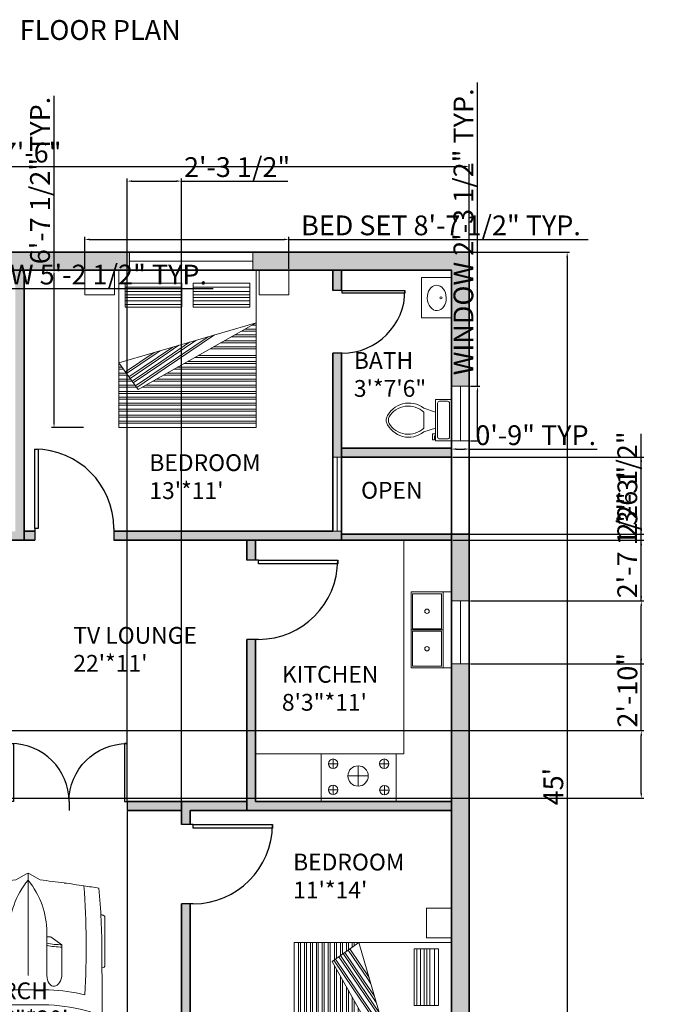
# Model space of a CAD drawing. Units: inches. Extents: x 1698 to 2352, y 1975 to 2732.
# Tile 4 of 4: x 2029 to 2352, y 2234 to 2732. Entities that reach past the tile are written whole.
import ezdxf

# ---------------------------------------------------------------- set-up
doc = ezdxf.new("R2010")
doc.units = ezdxf.units.IN
for name, color, linetype, lineweight in [('A-ANNO-DIMS', 2, 'Continuous', 18), ('A-ANNO-TEXT', 7, 'Continuous', 25), ('A-AREA-IDEN', 7, 'Continuous', 18), ('A-EQPM', 10, 'Continuous', 18), ('A-FLOR-CASE', 9, 'Continuous', 18), ('A-FLOR-FIXT', 231, 'Continuous', 18), ('A-WALL-PATT', 52, 'Continuous', 13), ('car', 171, 'Continuous', 13), ('door', 80, 'Continuous', 25), ('fur', 10, 'Continuous', 18), ('wall', 7, 'Continuous', 35), ('window', 130, 'Continuous', 18)]:
    doc.layers.add(name, color=color, linetype=linetype, lineweight=lineweight)
doc.styles.get("Standard").update_dxf_attribs({"font": 'arial.ttf'})
doc.dimstyles.new('ISO-25', dxfattribs={"dimtxt": 10, "dimasz": 2.5, "dimexe": 1.25, "dimexo": 0.625, "dimtad": 1, "dimdec": 0, "dimlunit": 4, "dimtxsty": 'Standard', "dimcen": 2.5, "dimadec": 0, "dimazin": 0, "dimtfac": 1, "dimtdec": 0, "dimtmove": 0, "dimatfit": 3, "dimfxl": 1, "dimarcsym": 0})

# ---------------------------------------------------------------- blocks, each defined once
blk = doc.blocks.new('*U2')
for p, q in [((0, 0), (0, -6)), ((40, 0), (40, -6))]:
    blk.add_line(p, q)
blk.add_lwpolyline([(0, 0), (0, 40), (1.75, 40), (1.75, 0)], close=True)
blk.add_arc((0, 0), 40, 0, 90)
blk = doc.blocks.new('*U6')
for p, q in [((21.1, 37.41), (21.1, 36.83)), ((46.55, 38.89), (22.35, 38.89)), ((47.8, 37.39), (47.8, 37.41)), ((87.99, 31.87), (74.76, 35.92)), ((134.31, 35.6), (119.29, 31.78)), ((135.45, 37.07), (135.45, 37.41)), ((136.7, 38.89), (160.9, 38.89)), ((162.15, 37.41), (162.15, 36.77)), ((70.03, 31.54), (86.41, 29.35)), ((186.47, -33.5), (186.47, 33.5)), ((188.4, -32.76), (188.4, 32.76)), ((138.42, 29.35), (157.25, 29.35)), ((164.52, 26.39), (164.52, -26.39)), ((186.47, 29.35), (167.01, 29.35)), ((32.27, 11.63), (36.13, 17.17)), ((36.13, 17.17), (50.94, 17.17)), ((32.12, 9.51), (32.12, 11.15)), ((58.92, -10.77), (58.92, 10.77)), ((66.55, -10.53), (66.55, 10.53)), ((186.47, -10.53), (186.47, 10.53)), ((3.27, 6.13), (0.1, 0.41)), ((29.77, 9.51), (51.68, 9.51)), ((82.74, 8.5), (82.74, -8.5)), ((0, 0), (51.68, 0)), ((0.1, -0.41), (3.27, -6.13)), ((29.77, -9.51), (51.68, -9.51)), ((32.12, -9.51), (32.12, -11.15)), ((32.27, -11.63), (36.13, -17.17)), ((36.13, -17.17), (50.94, -17.17)), ((86.41, -29.35), (70.03, -31.54)), ((157.25, -29.35), (138.42, -29.35)), ((167.01, -29.35), (186.47, -29.35)), ((87.99, -31.87), (74.76, -35.92)), ((134.31, -35.6), (119.29, -31.78)), ((21.1, -37.41), (21.1, -36.83)), ((46.55, -38.89), (22.35, -38.89)), ((47.8, -37.39), (47.8, -37.41)), ((135.45, -37.07), (135.45, -37.41)), ((136.7, -38.89), (160.9, -38.89)), ((162.15, -37.41), (162.15, -36.77))]:
    blk.add_line(p, q)
for centre, major_axis, ratio, start_param, end_param in [((266.03, -27.52), (0, 313.31), 0.842304, 1.367076, 1.39176), ((41.19, -490.86), (0, 528.23), 0.842304, 0.00281, 0.075598), ((22.35, 37.41), (0, -1.48), 0.842304, 3.141593, 4.712389), ((64.48, -10555.62), (0, 10593.03), 0.842304, -0.013397, 0.002797), ((46.55, 37.41), (0, 1.48), 0.842304, -1.570796, 0), ((64.48, -10555.62), (0, -10591.55), 0.842304, 3.133765, 3.140441), ((136.7, 37.41), (0, -1.48), 0.842304, 3.141593, 4.712389), ((160.9, 37.41), (0, 1.48), 0.842304, -1.570796, 0), ((180.63, 35.84), (0, 2.22), 0.842304, -0.013017, 1.249894), ((64.48, -10556.36), (0, 10595.31), 0.842304, -0.013397, -0.013017), ((183.98, 33.5), (0, -2.96), 0.842304, 1.570796, 3.128196), ((183.98, 32.76), (0, -5.25), 0.842304, 1.570796, 3.128196), ((135.29, 5.39), (0, 81.77), 0.842304, 1.245306, 1.50788), ((95.79, -3666.35), (0, -3698.24), 0.842304, 3.134049, 3.144098), ((259.18, -27.52), (0, -305.3), 0.842304, 4.528606, 4.561838), ((37.47, -593.96), (0, -623.33), 0.842304, 3.096046, 3.200911), ((134.4, 5.39), (0, -89.78), 0.842304, 4.449482, 4.652344), ((149.6, 2.8), (0, -79.58), 0.842304, 4.372215, 4.640744), ((17.08, 0), (0, 147.02), 0.842304, 4.511394, 4.913384), ((35.91, 0), (0, 147.02), 0.842304, 4.511394, 4.913384), ((167.01, 26.39), (0, 2.96), 0.842304, 0, 1.570796), ((-204.49, 52.4), (0, -250.96), 0.842304, 1.385369, 1.434372), ((13.04, 17.01), (0, 27.42), 0.842304, 4.435146, 4.718221), ((14.2, 17.01), (0, 27.42), 0.842304, 4.435146, 4.718221), ((50.79, 13.34), (6.34, -0.36), 0.603834, -1.395552, 1.581315), ((32.75, 11.15), (0, 0.74), 0.842304, 0.879714, 1.570796), ((29.77, -46.66), (0, 56.17), 0.842304, 0, 0.590319), ((0.62, 0), (0, -0.74), 0.842304, 4.131459, 5.293319), ((29.77, 46.66), (0, 56.17), 0.842304, 2.551274, 3.141593), ((-204.49, -52.4), (0, 250.96), 0.842304, -1.434372, -1.385369), ((13.04, -17.01), (0, -27.42), 0.842304, 1.564964, 1.848039), ((14.2, -17.01), (0, -27.42), 0.842304, 1.564964, 1.848039), ((149.6, -2.8), (0, -79.58), 0.842304, -1.499151, -1.230623), ((32.75, -11.15), (0, -0.74), 0.842304, 4.712389, 5.403472), ((134.4, -5.39), (0, -89.78), 0.842304, -1.510751, -1.307889), ((135.29, -5.39), (0, -81.77), 0.842304, -1.50788, -1.245306), ((259.18, 27.52), (0, 305.3), 0.842304, 1.721348, 1.754579), ((266.03, 27.52), (0, 313.31), 0.842304, 1.749832, 1.774517), ((37.47, 593.96), (0, -623.33), 0.842304, -0.059319, 0.045547), ((167.01, -26.39), (0, -2.96), 0.842304, 4.712389, 6.283185), ((95.79, 3666.35), (0, -3698.24), 0.842304, -0.002505, 0.007544), ((183.98, -33.5), (0, 2.96), 0.842304, 3.15499, 4.712389), ((183.98, -32.76), (0, -5.25), 0.842304, 0.013397, 1.570796), ((41.19, 490.86), (0, -528.23), 0.842304, -0.075598, -0.00281), ((22.35, -37.41), (0, 1.48), 0.842304, 1.570796, 3.141593), ((64.48, 10555.62), (0, 10593.03), 0.842304, 3.138796, 3.15499), ((46.55, -37.41), (0, -1.48), 0.842304, 0, 1.570796), ((64.48, 10555.62), (0, -10591.55), 0.842304, 0.001152, 0.007828), ((136.7, -37.41), (0, -1.48), 0.842304, -1.570796, 0), ((160.9, -37.41), (0, 1.48), 0.842304, 3.141593, 4.712389), ((180.63, -35.84), (0, -2.22), 0.842304, -1.249894, 0.013017), ((64.48, 10556.36), (0, 10595.31), 0.842304, 3.15461, 3.15499)]:
    blk.add_ellipse(centre, major_axis=major_axis, ratio=ratio, start_param=start_param, end_param=end_param)
at = {"extrusion": (0, 0, -1)}
blk.add_ellipse((50.79, -13.34), major_axis=(6.34, 0.36), ratio=0.603834, start_param=-1.395552, end_param=1.581315, dxfattribs=at)
blk = doc.blocks.new('*U4')
for p, q in [((9.5, -6), (9.5, -2)), ((-10, -8.5), (-8, -8.5)), ((-10, -9.5), (-10, -8.5)), ((-7, -9.5), (-10, -9.5)), ((-8, -8.5), (-8, -8)), ((-7, -8), (-7, -9.5)), ((-4, -8), (-6, -14)), ((4, -8), (6, -14)), ((4, -14), (-4, -14))]:
    blk.add_line(p, q)
blk.add_lwpolyline([(10.5, -8), (10.5, 0), (-10.5, 0), (-10.5, -8)], close=True)
for points in [[(-9.5, -2), (-9.5, -6)], [(8.5, -1), (-8.5, -1)], [(-8.5, -7), (8.5, -7)]]:
    blk.add_lwpolyline(points)
for centre, radius, start, end in [((-8.62, -1.88), 0.884, 81.8699, 188.1301), ((8.62, -1.88), 0.884, 351.8699, 98.1301), ((-8.62, -6.12), 0.884, 171.8699, 278.1301), ((8.62, -6.12), 0.884, 261.8699, 8.1301), ((3.52, -21.58), 12.17, 141.4691, 247.9714), ((4.2, -21.82), 11.33, 136.3677, 238.9468), ((-3.52, -21.58), 12.17, 292.0284, 38.5307), ((-4.2, -21.82), 11.33, 301.053, 43.6321), ((0, -27.88), 4, 245.7318, 294.2682), ((0, -29), 4, 254.8605, 285.1395)]:
    blk.add_arc(centre, radius, start, end)
blk = doc.blocks.new('*D7')
at = {"layer": 'A-ANNO-DIMS', "color": 0, "lineweight": -2, "transparency": 16777216}
for p, q in [((1805.99, 2614.89), (1805.99, 2658.85)), ((1808.49, 2657.6), (2253.49, 2657.6)), ((2255.99, 2614.89), (2255.99, 2658.85))]:
    blk.add_line(p, q, dxfattribs=at)
at = {"layer": 'A-ANNO-DIMS', "color": 0, "lineweight": 100, "transparency": 16777216}
for points in [[(1808.49, 2658.02), (1808.49, 2657.18), (1805.99, 2657.6)], [(2253.49, 2658.02), (2253.49, 2657.18), (2255.99, 2657.6)]]:
    blk.add_solid(points, dxfattribs=at)
at = {"layer": 'Defpoints', "color": 0, "lineweight": 100, "transparency": 16777216}
for p in [(2255.99, 2657.6), (1805.99, 2614.26), (2255.99, 2614.26)]:
    blk.add_point(p, dxfattribs=at)
at = {"layer": 'A-ANNO-DIMS', "color": 0, "transparency": 16777216, "insert": (2030.99, 2663.33), "char_height": 10, "attachment_point": 5}
blk.add_mtext('37\'-6"', dxfattribs=at)
blk = doc.blocks.new('*D8')
at = {"layer": 'A-ANNO-DIMS', "color": 0, "lineweight": -2, "transparency": 16777216}
for p, q in [((2256.62, 2614.26), (2306.74, 2614.26)), ((2305.49, 2611.76), (2305.49, 2076.76)), ((2256.62, 2074.26), (2306.74, 2074.26))]:
    blk.add_line(p, q, dxfattribs=at)
at = {"layer": 'A-ANNO-DIMS', "color": 0, "lineweight": 100, "transparency": 16777216}
for points in [[(2305.07, 2611.76), (2305.9, 2611.76), (2305.49, 2614.26)], [(2305.07, 2076.76), (2305.9, 2076.76), (2305.49, 2074.26)]]:
    blk.add_solid(points, dxfattribs=at)
at = {"layer": 'Defpoints', "color": 0, "lineweight": 100, "transparency": 16777216}
for p in [(2255.99, 2614.26), (2255.99, 2074.26), (2305.49, 2074.26)]:
    blk.add_point(p, dxfattribs=at)
at = {"layer": 'A-ANNO-DIMS', "color": 0, "transparency": 16777216, "insert": (2299.78, 2344.26), "char_height": 10, "attachment_point": 5, "rotation": 90}
blk.add_mtext("45'", dxfattribs=at)
blk = doc.blocks.new('BED-DOUBLE-WITH-NIGHTSTANDS')
for p, q in [((20.55, 70.98), (49.18, 70.98)), ((54.81, 70.98), (83.45, 70.98)), ((20.55, 67.05), (49.18, 67.05)), ((20.55, 65.74), (49.18, 65.74)), ((20.61, 68.69), (49.25, 68.69)), ((54.81, 67.05), (83.45, 67.05)), ((54.81, 65.74), (83.45, 65.74)), ((54.87, 68.69), (83.51, 68.69)), ((20.55, 63.98), (49.18, 63.98)), ((20.55, 62.15), (49.18, 62.15)), ((54.81, 63.98), (83.45, 63.98)), ((54.81, 62.15), (83.45, 62.15)), ((17.28, 32.76), (86.63, 52.89)), ((86.63, 52.89), (27, 19.28)), ((81.11, 49.78), (86.63, 49.78)), ((84.66, 51.78), (86.63, 51.78)), ((86.25, 52.78), (86.63, 52.78)), ((40.19, 30.78), (62.43, 45.87)), ((40.75, 29.96), (65.55, 46.77)), ((74.02, 45.78), (86.63, 45.78)), ((75.79, 46.78), (86.63, 46.78)), ((79.34, 48.78), (86.63, 48.78)), ((36.83, 35.44), (44.53, 40.67)), ((37.39, 34.62), (47.65, 41.57)), ((38.42, 33.24), (53.01, 43.13)), ((38.98, 32.41), (56.13, 44.04)), ((65.15, 40.78), (86.63, 40.78)), ((68.7, 42.78), (86.63, 42.78)), ((70.47, 43.78), (86.63, 43.78)), ((20.62, 28.13), (35.05, 37.91)), ((21.18, 27.3), (35.61, 37.09)), ((22.4, 25.66), (36.83, 35.44)), ((35.61, 37.09), (38.16, 38.82)), ((55.69, 35.45), (86.63, 35.45)), ((57.46, 36.45), (86.63, 36.45)), ((63.38, 39.78), (86.63, 39.78)), ((27, 19.28), (17.28, 32.76)), ((17.28, 32.45), (17.5, 32.45)), ((17.28, 30.45), (18.94, 30.45)), ((22.96, 24.83), (37.39, 34.62)), ((23.99, 23.45), (38.42, 33.24)), ((24.55, 22.62), (38.98, 32.41)), ((25.76, 21), (40.19, 30.78)), ((26.32, 20.17), (40.75, 29.96)), ((46.82, 30.45), (86.63, 30.45)), ((50.37, 32.45), (86.63, 32.45)), ((52.14, 33.45), (86.63, 33.45)), ((17.28, 29.45), (19.66, 29.45)), ((17.28, 27.45), (21.11, 27.45)), ((17.28, 26.45), (21.83, 26.45)), ((39.73, 26.45), (86.63, 26.45)), ((41.5, 27.45), (86.63, 27.45)), ((45.05, 29.45), (86.63, 29.45)), ((17.28, 24.45), (23.27, 24.45)), ((17.28, 23.45), (23.99, 23.45)), ((17.28, 21.45), (25.43, 21.45)), ((17.28, 20.45), (26.16, 20.45)), ((29.09, 20.45), (86.63, 20.45)), ((30.86, 21.45), (86.63, 21.45)), ((34.41, 23.45), (86.63, 23.45)), ((36.18, 24.45), (86.63, 24.45)), ((17.28, 18.28), (86.63, 18.28)), ((17.28, 17.28), (86.63, 17.28)), ((17.28, 15.28), (86.63, 15.28)), ((17.28, 14.28), (86.63, 14.28)), ((17.28, 12.28), (86.63, 12.28)), ((17.28, 11.28), (86.63, 11.28)), ((17.28, 9.28), (86.63, 9.28)), ((17.28, 8.28), (86.63, 8.28)), ((17.28, 6.28), (86.63, 6.28)), ((17.28, 5.28), (86.63, 5.28)), ((17.28, 3.28), (86.63, 3.28)), ((17.28, 2.28), (86.63, 2.28))]:
    blk.add_line(p, q)
for points in [[(0, 79.57), (15.07, 79.57), (15.07, 67), (0, 67)], [(17.28, 79.57), (86.63, 79.57), (86.63, 0), (17.28, 0)], [(88.18, 79.57), (103.25, 79.57), (103.25, 67), (88.18, 67)], [(20.55, 73), (49.18, 73), (49.18, 60.76), (20.55, 60.76)], [(54.81, 73), (83.45, 73), (83.45, 60.76), (54.81, 60.76)]]:
    blk.add_lwpolyline(points, close=True)
blk = doc.blocks.new('BASIN-VANITY')
blk.add_lwpolyline([(0, 20.39), (15.22, 20.39), (15.22, 0), (0, 0)], close=True)
blk.add_circle((5.32, 10.07), 0.551)
blk.add_ellipse((7.43, 9.98), major_axis=(-0.23, -6.4), ratio=0.75221)
blk = doc.blocks.new('WIN-BATH-27_578')
blk.add_line((4.5, 0), (4.5, 27.58))
blk.add_lwpolyline([(0, 0), (9, 0), (9, 27.58), (0, 27.58)], close=True)
blk = doc.blocks.new('WIN-BEDROOM-62_374')
blk.add_line((0, 4.5), (62.37, 4.5))
blk.add_lwpolyline([(0, 0), (62.37, 0), (62.37, 9), (0, 9)], close=True)
blk = doc.blocks.new('*D19')
at = {"layer": 'A-ANNO-DIMS', "color": 0, "lineweight": -2, "transparency": 16777216}
for p, q in [((2061.59, 2605.89), (2061.59, 2622)), ((2164.84, 2605.89), (2164.84, 2622)), ((2064.09, 2620.75), (2162.34, 2620.75)), ((2164.84, 2620.75), (2316.06, 2620.75))]:
    blk.add_line(p, q, dxfattribs=at)
at = {"layer": 'A-ANNO-DIMS', "color": 0, "lineweight": 100, "transparency": 16777216}
for points in [[(2064.09, 2621.17), (2064.09, 2620.33), (2061.59, 2620.75)], [(2162.34, 2621.17), (2162.34, 2620.33), (2164.84, 2620.75)]]:
    blk.add_solid(points, dxfattribs=at)
at = {"layer": 'Defpoints', "color": 0, "lineweight": 100, "transparency": 16777216}
for p in [(2164.84, 2620.75), (2061.59, 2605.26), (2164.84, 2605.26)]:
    blk.add_point(p, dxfattribs=at)
at = {"layer": 'A-ANNO-DIMS', "color": 0, "transparency": 16777216, "insert": (2241.7, 2626.55), "char_height": 10, "attachment_point": 5}
blk.add_mtext('BED SET 8\'-7 1/2" TYP.', dxfattribs=at)
blk = doc.blocks.new('*D20')
at = {"layer": 'A-ANNO-DIMS', "color": 0, "lineweight": -2, "transparency": 16777216}
for p, q in [((2046.1, 2605.26), (2046.1, 2693.32)), ((2060.97, 2605.26), (2044.85, 2605.26)), ((2046.1, 2528.19), (2046.1, 2602.76)), ((2060.97, 2525.69), (2044.85, 2525.69))]:
    blk.add_line(p, q, dxfattribs=at)
at = {"layer": 'A-ANNO-DIMS', "color": 0, "lineweight": 100, "transparency": 16777216}
for points in [[(2045.69, 2602.76), (2046.52, 2602.76), (2046.1, 2605.26)], [(2045.69, 2528.19), (2046.52, 2528.19), (2046.1, 2525.69)]]:
    blk.add_solid(points, dxfattribs=at)
at = {"layer": 'Defpoints', "color": 0, "lineweight": 100, "transparency": 16777216}
for p in [(2046.1, 2605.26), (2061.59, 2605.26), (2061.59, 2525.69)]:
    blk.add_point(p, dxfattribs=at)
at = {"layer": 'A-ANNO-DIMS', "color": 0, "transparency": 16777216, "insert": (2040.31, 2650.54), "char_height": 10, "attachment_point": 5, "rotation": 90}
blk.add_mtext('6\'-7 1/2" TYP.', dxfattribs=at)
blk = doc.blocks.new('*D27')
at = {"layer": 'A-ANNO-DIMS', "color": 0, "lineweight": -2, "transparency": 16777216}
for p, q in [((2260.13, 2546.53), (2260.13, 2700.13)), ((2256.62, 2546.53), (2261.38, 2546.53)), ((2260.13, 2521.45), (2260.13, 2544.03)), ((2256.62, 2518.95), (2261.38, 2518.95))]:
    blk.add_line(p, q, dxfattribs=at)
at = {"layer": 'A-ANNO-DIMS', "color": 0, "lineweight": 100, "transparency": 16777216}
for points in [[(2259.71, 2544.03), (2260.54, 2544.03), (2260.13, 2546.53)], [(2259.71, 2521.45), (2260.54, 2521.45), (2260.13, 2518.95)]]:
    blk.add_solid(points, dxfattribs=at)
at = {"layer": 'Defpoints', "color": 0, "lineweight": 100, "transparency": 16777216}
for p in [(2255.99, 2546.53), (2260.13, 2546.53), (2255.99, 2518.95)]:
    blk.add_point(p, dxfattribs=at)
at = {"layer": 'A-ANNO-DIMS', "color": 0, "transparency": 16777216, "insert": (2254.33, 2624.58), "char_height": 10, "attachment_point": 5, "rotation": 90}
blk.add_mtext('WINDOW 2\'-3 1/2" TYP.', dxfattribs=at)
blk = doc.blocks.new('*D28')
at = {"layer": 'A-ANNO-DIMS', "color": 0, "lineweight": -2, "transparency": 16777216}
for p, q in [((2246.99, 2518.33), (2246.99, 2513.57)), ((2255.99, 2518.33), (2255.99, 2513.57)), ((2249.49, 2514.82), (2253.49, 2514.82)), ((2255.99, 2514.82), (2320.7, 2514.82))]:
    blk.add_line(p, q, dxfattribs=at)
at = {"layer": 'A-ANNO-DIMS', "color": 0, "lineweight": 100, "transparency": 16777216}
for points in [[(2249.49, 2515.23), (2249.49, 2514.4), (2246.99, 2514.82)], [(2253.49, 2515.23), (2253.49, 2514.4), (2255.99, 2514.82)]]:
    blk.add_solid(points, dxfattribs=at)
at = {"layer": 'Defpoints', "color": 0, "lineweight": 100, "transparency": 16777216}
for p in [(2246.99, 2518.95), (2255.99, 2518.95), (2255.99, 2514.82)]:
    blk.add_point(p, dxfattribs=at)
at = {"layer": 'A-ANNO-DIMS', "color": 0, "transparency": 16777216, "insert": (2289.59, 2520.55), "char_height": 10, "attachment_point": 5}
blk.add_mtext('0\'-9" TYP.', dxfattribs=at)
blk = doc.blocks.new('*D29')
at = {"layer": 'A-ANNO-DIMS', "color": 0, "lineweight": -2, "transparency": 16777216}
for p, q in [((1910.52, 2604.64), (1910.52, 2594.66)), ((1972.89, 2604.64), (1972.89, 2594.66)), ((1913.02, 2595.91), (1970.39, 2595.91)), ((1972.89, 2595.91), (2126.48, 2595.91))]:
    blk.add_line(p, q, dxfattribs=at)
at = {"layer": 'A-ANNO-DIMS', "color": 0, "lineweight": 100, "transparency": 16777216}
for points in [[(1913.02, 2596.32), (1913.02, 2595.49), (1910.52, 2595.91)], [(1970.39, 2596.32), (1970.39, 2595.49), (1972.89, 2595.91)]]:
    blk.add_solid(points, dxfattribs=at)
at = {"layer": 'Defpoints', "color": 0, "lineweight": 100, "transparency": 16777216}
for p in [(1910.52, 2605.26), (1972.89, 2605.26), (1972.89, 2595.91)]:
    blk.add_point(p, dxfattribs=at)
at = {"layer": 'A-ANNO-DIMS', "color": 0, "transparency": 16777216, "insert": (2050.94, 2601.7), "char_height": 10, "attachment_point": 5}
blk.add_mtext('WINDOW 5\'-2 1/2" TYP.', dxfattribs=at)
blk = doc.blocks.new('*D37')
at = {"layer": 'A-ANNO-DIMS', "color": 0, "lineweight": -2, "transparency": 16777216}
for p, q in [((2024.3, 2331.64), (2024.3, 1983.28)), ((2083.04, 2331.64), (2083.04, 1983.28)), ((2026.8, 1984.53), (2080.54, 1984.53)), ((2083.04, 1984.53), (2144.84, 1984.53))]:
    blk.add_line(p, q, dxfattribs=at)
at = {"layer": 'A-ANNO-DIMS', "color": 0, "lineweight": 100, "transparency": 16777216}
for points in [[(2026.8, 1984.94), (2026.8, 1984.11), (2024.3, 1984.53)], [(2080.54, 1984.94), (2080.54, 1984.11), (2083.04, 1984.53)]]:
    blk.add_solid(points, dxfattribs=at)
at = {"layer": 'Defpoints', "color": 0, "lineweight": 100, "transparency": 16777216}
for p in [(2024.3, 2332.26), (2083.04, 2332.26), (2083.04, 1984.53)]:
    blk.add_point(p, dxfattribs=at)
at = {"layer": 'A-ANNO-DIMS', "color": 0, "transparency": 16777216, "insert": (2115.19, 1990.32), "char_height": 10, "attachment_point": 5}
blk.add_mtext('4\'-10 1/2"', dxfattribs=at)
blk = doc.blocks.new('*D38')
at = {"layer": 'A-ANNO-DIMS', "color": 0, "lineweight": -2, "transparency": 16777216}
for p, q in [((2083.04, 2337.39), (2083.04, 2651.46)), ((2085.54, 2650.21), (2107.99, 2650.21)), ((2110.49, 2332.89), (2110.49, 2651.46)), ((2110.49, 2650.21), (2164.3, 2650.21))]:
    blk.add_line(p, q, dxfattribs=at)
at = {"layer": 'A-ANNO-DIMS', "color": 0, "lineweight": 100, "transparency": 16777216}
for points in [[(2085.54, 2650.63), (2085.54, 2649.8), (2083.04, 2650.21)], [(2107.99, 2650.63), (2107.99, 2649.8), (2110.49, 2650.21)]]:
    blk.add_solid(points, dxfattribs=at)
at = {"layer": 'Defpoints', "color": 0, "lineweight": 100, "transparency": 16777216}
for p in [(2110.49, 2650.21), (2083.04, 2336.76), (2110.49, 2332.26)]:
    blk.add_point(p, dxfattribs=at)
at = {"layer": 'A-ANNO-DIMS', "color": 0, "transparency": 16777216, "insert": (2138.64, 2656.01), "char_height": 10, "attachment_point": 5}
blk.add_mtext('2\'-3 1/2"', dxfattribs=at)
blk = doc.blocks.new('*D45')
at = {"layer": 'A-ANNO-DIMS', "color": 0, "lineweight": -2, "transparency": 16777216}
for p, q in [((2342.94, 2372.57), (2342.94, 2410.85)), ((1871.12, 2372.57), (2344.19, 2372.57)), ((2342.94, 2340.87), (2342.94, 2370.07)), ((1871.12, 2338.37), (2344.19, 2338.37))]:
    blk.add_line(p, q, dxfattribs=at)
at = {"layer": 'A-ANNO-DIMS', "color": 0, "lineweight": 100, "transparency": 16777216}
for points in [[(2342.52, 2370.07), (2343.36, 2370.07), (2342.94, 2372.57)], [(2342.52, 2340.87), (2343.36, 2340.87), (2342.94, 2338.37)]]:
    blk.add_solid(points, dxfattribs=at)
at = {"layer": 'Defpoints', "color": 0, "lineweight": 100, "transparency": 16777216}
for p in [(1870.49, 2372.57), (2342.94, 2372.57), (1870.49, 2338.37)]:
    blk.add_point(p, dxfattribs=at)
at = {"layer": 'A-ANNO-DIMS', "color": 0, "transparency": 16777216, "insert": (2337.21, 2392.96), "char_height": 10, "attachment_point": 5, "rotation": 90}
blk.add_mtext('2\'-10"', dxfattribs=at)
blk = doc.blocks.new('*D47')
at = {"layer": 'A-ANNO-DIMS', "color": 0, "lineweight": -2, "transparency": 16777216}
for p, q in [((2247.62, 2510.76), (2344.19, 2510.76)), ((2342.94, 2474.26), (2342.94, 2508.26)), ((2247.62, 2471.76), (2344.19, 2471.76))]:
    blk.add_line(p, q, dxfattribs=at)
at = {"layer": 'A-ANNO-DIMS', "color": 0, "lineweight": 100, "transparency": 16777216}
for points in [[(2342.52, 2508.26), (2343.36, 2508.26), (2342.94, 2510.76)], [(2342.52, 2474.26), (2343.36, 2474.26), (2342.94, 2471.76)]]:
    blk.add_solid(points, dxfattribs=at)
at = {"layer": 'Defpoints', "color": 0, "lineweight": 100, "transparency": 16777216}
for p in [(2246.99, 2510.76), (2342.94, 2510.76), (2246.99, 2471.76)]:
    blk.add_point(p, dxfattribs=at)
at = {"layer": 'A-ANNO-DIMS', "color": 0, "transparency": 16777216, "insert": (2337.21, 2491.26), "char_height": 10, "attachment_point": 5, "rotation": 90}
blk.add_mtext('3\'-3"', dxfattribs=at)
blk = doc.blocks.new('*D48')
at = {"layer": 'A-ANNO-DIMS', "color": 0, "lineweight": -2, "transparency": 16777216}
for p, q in [((2342.94, 2438.09), (2342.94, 2491.9)), ((2256.62, 2438.09), (2344.19, 2438.09)), ((2342.94, 2408.87), (2342.94, 2435.59)), ((2256.62, 2406.37), (2344.19, 2406.37))]:
    blk.add_line(p, q, dxfattribs=at)
at = {"layer": 'A-ANNO-DIMS', "color": 0, "lineweight": 100, "transparency": 16777216}
for points in [[(2342.52, 2435.59), (2343.36, 2435.59), (2342.94, 2438.09)], [(2342.52, 2408.87), (2343.36, 2408.87), (2342.94, 2406.37)]]:
    blk.add_solid(points, dxfattribs=at)
at = {"layer": 'Defpoints', "color": 0, "lineweight": 100, "transparency": 16777216}
for p in [(2255.99, 2438.09), (2342.94, 2438.09), (2255.99, 2406.37)]:
    blk.add_point(p, dxfattribs=at)
at = {"layer": 'A-ANNO-DIMS', "color": 0, "transparency": 16777216, "insert": (2337.15, 2466.25), "char_height": 10, "attachment_point": 5, "rotation": 90}
blk.add_mtext('2\'-7 1/2"', dxfattribs=at)
blk = doc.blocks.new('*D49')
at = {"layer": 'A-ANNO-DIMS', "color": 0, "lineweight": -2, "transparency": 16777216}
for p, q in [((2342.94, 2468.76), (2342.94, 2522.57)), ((2247.62, 2468.76), (2344.19, 2468.76)), ((2342.94, 2440.59), (2342.94, 2466.26)), ((2256.62, 2438.09), (2344.19, 2438.09))]:
    blk.add_line(p, q, dxfattribs=at)
at = {"layer": 'A-ANNO-DIMS', "color": 0, "lineweight": 100, "transparency": 16777216}
for points in [[(2342.52, 2466.26), (2343.36, 2466.26), (2342.94, 2468.76)], [(2342.52, 2440.59), (2343.36, 2440.59), (2342.94, 2438.09)]]:
    blk.add_solid(points, dxfattribs=at)
at = {"layer": 'Defpoints', "color": 0, "lineweight": 100, "transparency": 16777216}
for p in [(2246.99, 2468.76), (2342.94, 2468.76), (2255.99, 2438.09)]:
    blk.add_point(p, dxfattribs=at)
at = {"layer": 'A-ANNO-DIMS', "color": 0, "transparency": 16777216, "insert": (2337.15, 2496.91), "char_height": 10, "attachment_point": 5, "rotation": 90}
blk.add_mtext('2\'-6 1/2"', dxfattribs=at)

msp = doc.modelspace()

# ---------------------------------------------------------------- hatches: boundary and pattern name
at = {"layer": 'A-WALL-PATT'}
h = msp.add_hatch(color=256, dxfattribs=at)
h.dxf.hatch_style = 1
h.paths.add_polyline_path([(1910.52, 2614.26), (1805.99, 2614.26), (1805.99, 2549.47), (1814.99, 2549.47), (1814.99, 2605.26), (1910.52, 2605.26)])
h.paths.add_polyline_path([(2084.19, 2614.26), (1972.89, 2614.26), (1972.89, 2605.26), (2026.49, 2605.26), (2084.19, 2605.26)])
h.paths.add_polyline_path([(2255.99, 2614.26), (2146.56, 2614.26), (2146.56, 2605.26), (2148.21, 2605.26), (2186.99, 2605.26), (2246.99, 2605.26), (2246.99, 2546.53), (2255.99, 2546.53)])
h.paths.add_polyline_path([(2191.49, 2605.26), (2186.99, 2605.26), (2186.99, 2595.02), (2191.49, 2595.02)], flags=17)
h.paths.add_polyline_path([(2191.49, 2563.28), (2186.99, 2563.28), (2186.99, 2510.76), (2191.49, 2510.76)])
h.paths.add_polyline_path([(2246.99, 2515.26), (2191.49, 2515.26), (2191.49, 2510.76), (2246.99, 2510.76)])
h.paths.add_polyline_path([(2030.99, 2605.26), (2026.49, 2605.26), (2026.49, 2473.26), (2020.85, 2473.26), (2020.85, 2468.76), (2030.99, 2468.76)])
h.paths.add_polyline_path([(1980.85, 2473.26), (1870.49, 2473.26), (1865.99, 2473.26), (1865.99, 2468.76), (1980.85, 2468.76)])
h.paths.add_polyline_path([(1828.36, 2413.26), (1814.99, 2413.26), (1814.99, 2408.76), (1828.36, 2408.76)])
h.paths.add_polyline_path([(1865.99, 2413.26), (1847.77, 2413.26), (1847.77, 2408.76), (1865.99, 2408.76)])
h.paths.add_polyline_path([(1870.49, 2418.36), (1865.99, 2418.36), (1865.99, 2372.57), (1870.49, 2372.57)])
h.paths.add_polyline_path([(2036.32, 2473.26), (2030.99, 2473.26), (2030.99, 2468.76), (2036.32, 2468.76)])
h.paths.add_polyline_path([(2191.49, 2473.26), (2186.99, 2473.26), (2076.32, 2473.26), (2076.32, 2468.76), (2191.49, 2468.76)])
h.paths.add_polyline_path([(2246.99, 2471.76), (2191.49, 2471.76), (2191.49, 2468.76), (2246.99, 2468.76)])
h.paths.add_polyline_path([(2255.99, 2406.37), (2246.99, 2406.37), (2246.99, 2404.25), (2246.99, 2336.76), (2246.99, 2083.26), (2127.92, 2083.26), (2127.92, 2074.26), (2255.99, 2074.26)])
h.paths.add_polyline_path([(2110.49, 2336.76), (2083.04, 2336.76), (2083.04, 2336.67), (2083.04, 2332.26), (2110.49, 2332.26)])
h.paths.add_polyline_path([(2024.3, 2336.76), (2003.04, 2336.76), (2003.04, 2332.26), (2024.3, 2332.26)])
h.paths.add_polyline_path([(2246.99, 2164.26), (2216.76, 2164.26), (2216.76, 2155.26), (2246.99, 2155.26)], flags=17)
h.paths.add_polyline_path([(1958.99, 2083.26), (1927.89, 2083.26), (1927.89, 2074.26), (1958.99, 2074.26)])
h.paths.add_polyline_path([(1963.49, 2185.34), (1958.99, 2185.34), (1958.99, 2083.26), (1963.49, 2083.26)])
h.paths.add_polyline_path([(1963.49, 2238.76), (1855.03, 2238.76, -0.010403), (1855.05, 2237.79), (1855.05, 2234.26), (1958.99, 2234.26), (1958.99, 2225.34), (1963.49, 2225.34)])
h.paths.add_polyline_path([(1831.56, 2237.79), (1831.56, 2238.76), (1814.99, 2238.76), (1814.99, 2234.26), (1831.56, 2234.26)])
h.paths.add_polyline_path([(1939.87, 2336.76), (1814.99, 2336.76), (1814.99, 2332.26), (1856.99, 2332.26), (1939.87, 2332.26)])
h.paths.add_polyline_path([(1814.99, 2377.93), (1805.99, 2377.93), (1805.99, 2325.81), (1814.99, 2325.81)])
h.paths.add_polyline_path([(1829.84, 2521.26), (1814.99, 2521.26), (1814.99, 2516.76), (1829.84, 2516.76)])
h.paths.add_polyline_path([(2255.99, 2471.76), (2246.99, 2471.76), (2246.99, 2438.09), (2255.99, 2438.09)])
h = msp.add_hatch(color=256, dxfattribs=at)
h.dxf.hatch_style = 1
h.paths.add_polyline_path([(1870.49, 2565.42), (1865.99, 2565.42), (1865.99, 2521.26), (1849.25, 2521.26), (1849.25, 2516.76), (1870.49, 2516.76)])
h.paths.add_polyline_path([(1870.49, 2605.26), (1865.99, 2605.26), (1865.99, 2598.8), (1870.49, 2598.8)])
h.paths.add_polyline_path([(2246.99, 2336.76), (2147.99, 2336.76), (2147.99, 2360.76), (2147.99, 2418.65), (2143.49, 2418.65), (2143.49, 2332.26), (2246.99, 2332.26)])
h.paths.add_polyline_path([(2143.49, 2336.76), (2110.49, 2336.76), (2110.49, 2325.07), (2114.99, 2325.07), (2114.99, 2332.26), (2143.49, 2332.26)])
h.paths.add_polyline_path([(2114.99, 2285.07), (2110.49, 2285.07), (2110.49, 2155.26), (2141.76, 2155.26), (2141.76, 2164.26), (2114.99, 2164.26)])
h.paths.add_polyline_path([(1814.99, 2298.28), (1805.99, 2298.28), (1805.99, 2074.26), (1852.89, 2074.26), (1852.89, 2083.26), (1814.99, 2083.26)])
h = msp.add_hatch(color=256, dxfattribs=at)
h.dxf.hatch_style = 1
h.paths.add_polyline_path([(2147.99, 2468.76), (2143.49, 2468.76), (2143.49, 2458.65), (2147.99, 2458.65)])

# ---------------------------------------------------------------- linework, layer by layer
at = {"layer": 'A-EQPM'}
for p, q in [((2189.51, 2355.85), (2184.76, 2355.85)), ((2187.14, 2355.85), (2187.14, 2358.23)), ((2187.14, 2358.23), (2187.14, 2353.47)), ((2187.14, 2353.47), (2187.14, 2355.85)), ((2187.14, 2355.85), (2189.51, 2355.85)), ((2199.8, 2349.64), (2199.8, 2354.78)), ((2199.8, 2354.78), (2199.8, 2344.5)), ((2213.01, 2355.85), (2210.63, 2355.85)), ((2210.63, 2355.85), (2215.38, 2355.85)), ((2213.01, 2355.85), (2213.01, 2358.23)), ((2213.01, 2358.23), (2213.01, 2353.47)), ((2213.01, 2353.47), (2213.01, 2355.85)), ((2199.8, 2349.64), (2194.66, 2349.64)), ((2194.66, 2349.64), (2204.94, 2349.64)), ((2199.8, 2344.5), (2199.8, 2349.64)), ((2187.14, 2345.04), (2187.14, 2340.28)), ((2213.08, 2342.51), (2213.08, 2344.88)), ((2213.08, 2344.88), (2213.08, 2340.13)), ((2189.51, 2342.66), (2184.76, 2342.66)), ((2187.14, 2340.28), (2187.14, 2342.66)), ((2187.14, 2342.66), (2189.51, 2342.66)), ((2213.08, 2342.51), (2210.71, 2342.51)), ((2210.71, 2342.51), (2215.46, 2342.51)), ((2213.08, 2340.13), (2213.08, 2342.51))]:
    msp.add_line(p, q, dxfattribs=at)
msp.add_lwpolyline([(2181.07, 2360.76), (2218.99, 2360.76), (2218.99, 2336.76), (2181.07, 2336.76)], close=True, dxfattribs=at)
for centre, radius in [((2187.14, 2355.85), 2.38), ((2199.8, 2349.64), 5.14), ((2213.01, 2355.85), 2.38), ((2187.14, 2342.66), 2.38), ((2213.08, 2342.51), 2.38)]:
    msp.add_circle(centre, radius, dxfattribs=at)
at = {"layer": 'A-FLOR-CASE'}
for p, q in [((2246.99, 2468.76), (2222.99, 2468.76)), ((2222.99, 2468.76), (2222.99, 2360.76)), ((2147.99, 2336.76), (2147.99, 2360.76)), ((2147.99, 2360.76), (2222.99, 2360.76))]:
    msp.add_line(p, q, dxfattribs=at)
at = {"layer": 'A-FLOR-FIXT'}
for p, q in [((2242.81, 2442.71), (2242.81, 2404.25)), ((2226.57, 2423.48), (2242.81, 2423.48))]:
    msp.add_line(p, q, dxfattribs=at)
for points in [[(2246.99, 2442.71), (2226.57, 2442.71), (2226.57, 2404.25), (2246.99, 2404.25)], [(2227.35, 2424.02), (2241.9, 2424.02), (2241.9, 2441.72), (2227.35, 2441.72)], [(2227.35, 2405.07), (2241.9, 2405.07), (2241.9, 2422.78), (2227.35, 2422.78)]]:
    msp.add_lwpolyline(points, close=True, dxfattribs=at)
for centre in [(2234.62, 2432.87), (2234.62, 2413.92)]:
    msp.add_circle(centre, 1.11, dxfattribs=at)
at = {"layer": 'wall'}
for p, q in [((2030.99, 2605.26), (2030.99, 2468.76)), ((2030.99, 2605.26), (2186.99, 2605.26)), ((2186.99, 2605.26), (2186.99, 2595.02)), ((2191.49, 2605.26), (2191.49, 2595.02)), ((2191.49, 2605.26), (2239.49, 2605.26)), ((2191.49, 2605.26), (2191.49, 2595.02)), ((2239.49, 2605.26), (2242.49, 2605.26)), ((2186.99, 2563.28), (2186.99, 2473.26)), ((2191.49, 2563.28), (2191.49, 2515.26)), ((2191.49, 2563.28), (2191.49, 2468.76)), ((2191.49, 2515.26), (2246.99, 2515.26)), ((2191.49, 2510.76), (2246.99, 2510.76)), ((2036.32, 2473.26), (2030.99, 2473.26)), ((2186.99, 2473.26), (2076.32, 2473.26)), ((2030.99, 2468.76), (2020.85, 2468.76)), ((2036.32, 2468.76), (2030.99, 2468.76)), ((2191.49, 2468.76), (2076.32, 2468.76)), ((2143.49, 2458.65), (2143.49, 2468.76)), ((2147.99, 2458.65), (2147.99, 2468.76)), ((2191.49, 2471.76), (2246.99, 2471.76)), ((2191.49, 2468.76), (2246.99, 2468.76)), ((2246.99, 2471.76), (2255.99, 2471.76)), ((2246.99, 2468.76), (2246.99, 2336.76)), ((2143.49, 2332.26), (2143.49, 2418.65)), ((2147.99, 2336.76), (2147.99, 2418.65)), ((2110.49, 2336.76), (2083.04, 2336.76)), ((2110.49, 2336.76), (2143.49, 2336.76)), ((2110.49, 2325.07), (2110.49, 2336.76)), ((2246.99, 2336.76), (2147.99, 2336.76)), ((2110.49, 2332.26), (2083.04, 2332.26)), ((2114.99, 2332.26), (2143.49, 2332.26)), ((2114.99, 2325.07), (2114.99, 2332.26)), ((2246.99, 2332.26), (2143.49, 2332.26)), ((2246.99, 2332.26), (2246.99, 2164.26)), ((2110.49, 2155.26), (2110.49, 2285.07)), ((2114.99, 2164.26), (2114.99, 2285.07))]:
    msp.add_line(p, q, dxfattribs=at)
for points in [[(2127.92, 2074.26), (2255.99, 2074.26), (2255.99, 2614.26), (1805.99, 2614.26), (1805.99, 2074.26), (1958.99, 2074.26)], [(2127.92, 2083.26), (2246.99, 2083.26), (2246.99, 2605.26), (1814.99, 2605.26), (1814.99, 2516.76)]]:
    msp.add_lwpolyline(points, dxfattribs=at)
at = {"layer": 'window'}
for p, q in [((2189.24, 2473.26), (2189.24, 2510.76)), ((2251.49, 2406.37), (2251.49, 2438.09))]:
    msp.add_line(p, q, dxfattribs=at)
for points in [[(2186.99, 2473.26), (2191.49, 2473.26), (2191.49, 2510.76), (2186.99, 2510.76)], [(2246.99, 2438.09), (2255.99, 2438.09), (2255.99, 2406.37), (2246.99, 2406.37)]]:
    msp.add_lwpolyline(points, close=True, dxfattribs=at)

# ---------------------------------------------------------------- block references
at = {"layer": 'A-FLOR-FIXT', "extrusion": (0, 0, -1), "zscale": -1}
msp.add_blockref('BASIN-VANITY', (-2246.99, 2581.2), dxfattribs=at)
at = {"layer": 'A-FLOR-FIXT', "xscale": -1, "rotation": 270}
msp.add_blockref('*U4', (2246.99, 2529.45), dxfattribs=at)
at = {"layer": 'car', "rotation": 270}
msp.add_blockref('*U6', (2032.95, 2300.49), dxfattribs=at)
at = {"layer": 'door', "xscale": 0.7935940236748947, "yscale": 0.7935940236748947, "zscale": 0.7935940236748947, "rotation": 270}
msp.add_blockref('*U2', (2191.75, 2595.02), dxfattribs=at)
at = {"layer": 'door'}
msp.add_blockref('*U2', (2036.32, 2474.76), dxfattribs=at)
at = {"layer": 'door', "rotation": 270}
for p in [(2149.49, 2458.65), (2116.49, 2325.07)]:
    msp.add_blockref('*U2', p, dxfattribs=at)
at = {"layer": 'door', "yscale": 0.734231061655472, "zscale": 0.734231061655472}
for p, xscale in [((2024.3, 2336.67), 0.734231061655472), ((2083.04, 2336.67), -0.734231061655472)]:
    msp.add_blockref('*U2', p, dxfattribs=dict(at, xscale=xscale))
at = {"layer": 'fur'}
msp.add_blockref('BED-DOUBLE-WITH-NIGHTSTANDS', (2061.59, 2525.69), dxfattribs=at)
at = {"layer": 'fur', "rotation": 270.0000000000057}
msp.add_blockref('BED-DOUBLE-WITH-NIGHTSTANDS', (2167.42, 2282.85), dxfattribs=at)
at = {"layer": 'window'}
for name, p in [('WIN-BEDROOM-62_374', (2084.19, 2605.26)), ('WIN-BATH-27_578', (2246.99, 2518.95))]:
    msp.add_blockref(name, p, dxfattribs=at)

# ---------------------------------------------------------------- texts
at = {"layer": 'A-ANNO-TEXT', "insert": (1974.3, 2731.6), "char_height": 10.0406, "attachment_point": 1}
msp.add_mtext_dynamic_manual_height_columns('GRIUND FLOOR PLAN', width=1490.6775, gutter_width=50.2, heights=[0], dxfattribs=at)
at = {"layer": 'A-AREA-IDEN', "char_height": 8.476, "attachment_point": 1}
for s, insert in [('BATH\\P3\'*7\'6"', (2197.66, 2563.83)), ("BEDROOM\\P13'*11'", (2094.28, 2512.19)), ('OPEN', (2201.3, 2498.24)), ("TV LOUNGE\\P22'*11'", (2055.85, 2424.93)), ('KITCHEN\\P8\'3"*11\'', (2161.28, 2405.22)), ("BEDROOM\\P11'*14'", (2166.97, 2310.37)), ('PORCH\\P11\'6"*20\'', (2003.94, 2245.32))]:
    msp.add_mtext_dynamic_manual_height_columns(s, width=272.6258, gutter_width=42.38, heights=[0], dxfattribs=dict(at, insert=insert))

# ---------------------------------------------------------------- dimensions: what is measured, and where the dimension line sits
at = {"layer": 'A-ANNO-DIMS'}
for base, p1, p2, text, picture, middle in [((2260.13, 2546.53), (2255.99, 2518.95), (2255.99, 2546.53), 'WINDOW <> TYP.', '*D27', (2254.33, 2624.58)), ((2046.1, 2605.26), (2061.59, 2525.69), (2061.59, 2605.26), '<> TYP.', '*D20', (2040.31, 2650.54))]:
    dim = msp.add_linear_dim(base=base, p1=p1, p2=p2, angle=90, text=text, dimstyle='ISO-25', override={"dimdec": 1, "dimlfac": 1, "dimrnd": 0, "dimzin": 1, "dimdsep": 46, "dimlunit": 4, "dimfrac": 2}, dxfattribs=at)
    dim.commit()
    dim.dimension.update_dxf_attribs({"geometry": picture, "text_midpoint": middle})
for base, p1, p2, override, picture, middle in [((2255.99, 2657.6), (1805.99, 2614.26), (2255.99, 2614.26), {"dimclrd": 0, "dimclre": 0, "dimclrt": 0}, '*D7', (2030.99, 2663.33)), ((2110.4914, 2650.2121), (2083.0375, 2336.7621), (2110.4914, 2332.2621), {"dimdec": 1, "dimlfac": 1, "dimrnd": 0, "dimzin": 1, "dimdsep": 46, "dimlunit": 4, "dimfrac": 2}, '*D38', (2138.6437, 2656.0111)), ((2083.04, 1984.53), (2024.3, 2332.26), (2083.04, 2332.26), {"dimdec": 1, "dimlfac": 1, "dimrnd": 0, "dimzin": 1, "dimdsep": 46, "dimlunit": 4, "dimfrac": 2}, '*D37', (2115.19, 1990.32))]:
    dim = msp.add_linear_dim(base=base, p1=p1, p2=p2, dimstyle='ISO-25', override=override, dxfattribs=at)
    dim.commit()
    dim.dimension.update_dxf_attribs({"geometry": picture, "text_midpoint": middle})
for base, p1, p2, text, picture, middle in [((2164.8417, 2620.7498), (2061.5902, 2605.2621), (2164.8417, 2605.2621), 'BED SET <> TYP.', '*D19', (2241.7013, 2626.5454)), ((1972.89, 2595.91), (1910.52, 2605.26), (1972.89, 2605.26), 'WINDOW <> TYP.', '*D29', (2050.94, 2601.7)), ((2255.99, 2514.82), (2246.99, 2518.95), (2255.99, 2518.95), '<> TYP.', '*D28', (2289.59, 2520.55))]:
    dim = msp.add_linear_dim(base=base, p1=p1, p2=p2, text=text, dimstyle='ISO-25', override={"dimdec": 1, "dimlfac": 1, "dimrnd": 0, "dimzin": 1, "dimdsep": 46, "dimlunit": 4, "dimfrac": 2}, dxfattribs=at)
    dim.commit()
    dim.dimension.update_dxf_attribs({"geometry": picture, "text_midpoint": middle})
for base, p1, p2, override, picture, middle in [((2305.49, 2074.26), (2255.99, 2614.26), (2255.99, 2074.26), {"dimclrd": 0, "dimclre": 0, "dimclrt": 0}, '*D8', (2299.78, 2344.26)), ((2342.94, 2468.76), (2255.99, 2438.09), (2246.99, 2468.76), {"dimdec": 1, "dimlfac": 1, "dimrnd": 0, "dimzin": 1, "dimdsep": 46, "dimlunit": 4, "dimfrac": 2}, '*D49', (2337.15, 2496.91)), ((2342.94, 2510.76), (2246.99, 2471.76), (2246.99, 2510.76), {"dimdec": 1, "dimlfac": 1, "dimrnd": 0, "dimzin": 1, "dimdsep": 46, "dimlunit": 4, "dimfrac": 2}, '*D47', (2337.21, 2491.26)), ((2342.94, 2438.09), (2255.99, 2406.37), (2255.99, 2438.09), {"dimdec": 1, "dimlfac": 1, "dimrnd": 0, "dimzin": 1, "dimdsep": 46, "dimlunit": 4, "dimfrac": 2}, '*D48', (2337.15, 2466.25)), ((2342.94, 2372.57), (1870.49, 2338.37), (1870.49, 2372.57), {"dimdec": 1, "dimlfac": 1, "dimrnd": 0, "dimzin": 1, "dimdsep": 46, "dimlunit": 4, "dimfrac": 2}, '*D45', (2337.21, 2392.96))]:
    dim = msp.add_linear_dim(base=base, p1=p1, p2=p2, angle=90, dimstyle='ISO-25', override=override, dxfattribs=at)
    dim.commit()
    dim.dimension.update_dxf_attribs({"geometry": picture, "text_midpoint": middle})

doc.saveas('drawing.dxf')
